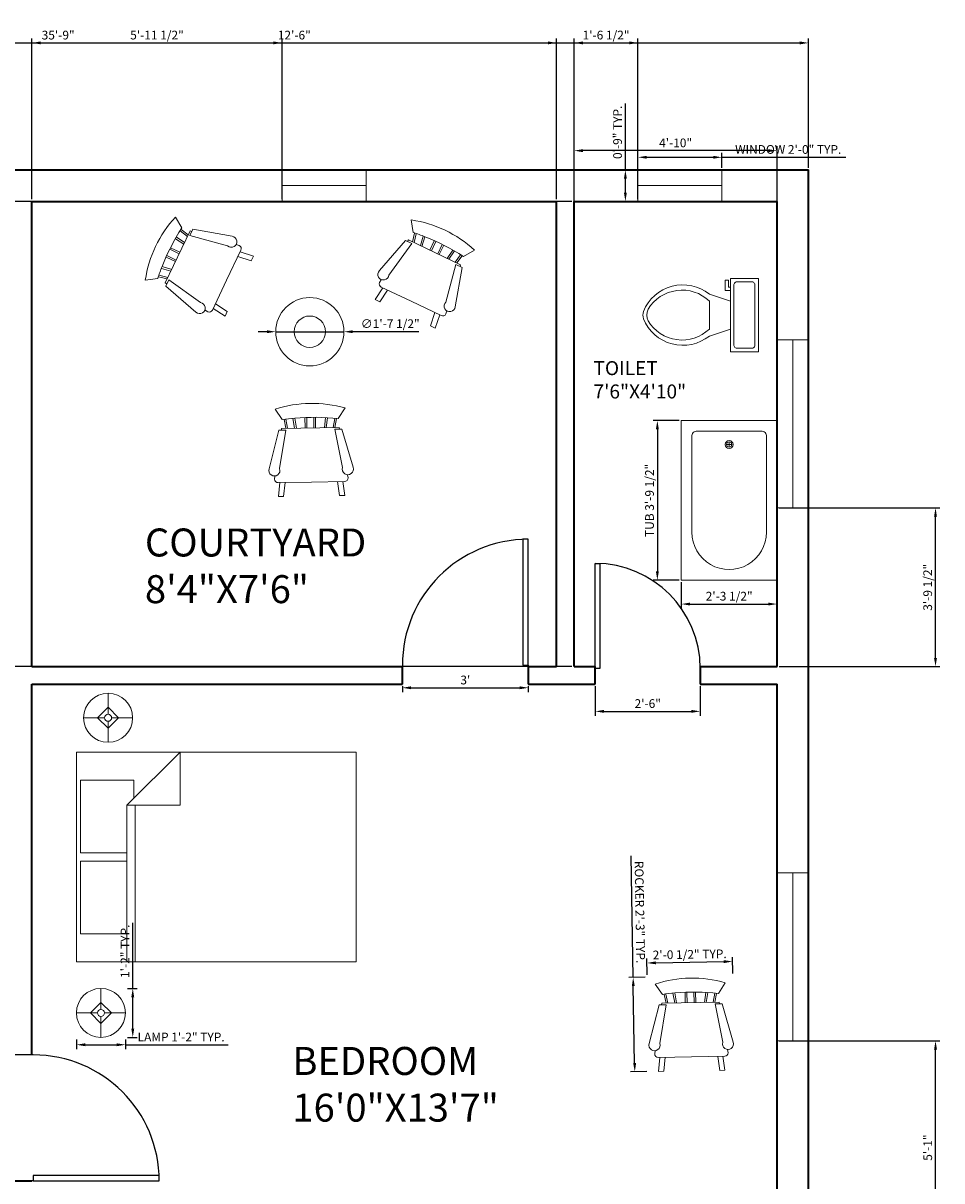
# Model space of a CAD drawing. Units: inches. Extents: x 3715 to 4224, y 2597 to 3354.
# Tile 5 of 5: x 3961 to 4224, y 3023 to 3354. Entities that reach past the tile are written whole.
import ezdxf

# ---------------------------------------------------------------- set-up
doc = ezdxf.new("R2010")
doc.units = ezdxf.units.IN
for name, color, linetype, lineweight in [('A-AREA-IDEN', 4, 'Continuous', 25), ('A-FLOR-FIXT', 9, 'Continuous', 18), ('A-WALL', 7, 'Continuous', 35), ('DIM', 1, 'Continuous', 18), ('DOOR', 3, 'Continuous', 25), ('FURNITURES', 30, 'Continuous', 18), ('WINDOW', 6, 'Continuous', 20)]:
    doc.layers.add(name, color=color, linetype=linetype, lineweight=lineweight)
doc.styles.get("Standard").update_dxf_attribs({"font": 'arial.ttf'})
doc.dimstyles.new('ISO-25', dxfattribs={"dimtxt": 2.5, "dimasz": 2.5, "dimexe": 1.25, "dimexo": 0.625, "dimtad": 1, "dimlunit": 3, "dimtxsty": 'Standard', "dimcen": 2.5, "dimadec": 0, "dimazin": 0, "dimtfac": 1, "dimtmove": 0, "dimatfit": 3, "dimfxl": 1, "dimarcsym": 0})

# ---------------------------------------------------------------- blocks, each defined once
blk = doc.blocks.new('*U4')
for p, q in [((0, 0), (0, -6)), ((-40, 0), (-40, -6))]:
    blk.add_line(p, q)
blk.add_lwpolyline([(0, 0), (0, 40), (-1.75, 40), (-1.75, 0)], close=True)
blk.add_arc((0, 0), 40, 90, 180)
blk = doc.blocks.new('*U2')
for p, q in [((0, 0), (0, -6)), ((40, 0), (40, -6))]:
    blk.add_line(p, q)
blk.add_lwpolyline([(0, 0), (0, 40), (1.75, 40), (1.75, 0)], close=True)
blk.add_arc((0, 0), 40, 0, 90)
blk = doc.blocks.new('Bed - Queen')
for p, q in [((0, -80.00003), (0, 0)), ((0, 0), (59.99999, 0)), ((59.99999, 0), (59.99999, -80.00003)), ((7.99999, -1.2), (28.79998, -1.2)), ((7.99999, -14.4), (7.99999, -1.2)), ((28.79998, -1.2), (28.79998, -14.4)), ((31.19999, -1.2), (51.99999, -1.2)), ((31.19999, -14.4), (31.19999, -1.2)), ((51.99999, -1.2), (51.99999, -16.4)), ((0, -14.4), (44.8, -14.4)), ((59.99999, -29.6), (44.8, -14.4)), ((44.8, -14.4), (44.8, -29.6)), ((51.99999, -16.4), (46.79936, -16.4)), ((44.8, -16.8), (0, -16.8)), ((44.8, -29.6), (59.99999, -29.6)), ((59.99999, -80.00003), (0, -80.00003))]:
    blk.add_line(p, q)
blk = doc.blocks.new('Lamp - Table')
for p, q in [((0, 7), (0, 1)), ((-1, 0), (-7, 0)), ((0, 3), (-3, 0)), ((-3, 0), (0, -3)), ((3, 0), (0, 3)), ((0, -3), (3, 0)), ((1, 0), (7, 0)), ((0, -1), (0, -7))]:
    blk.add_line(p, q)
for radius in [7, 1]:
    blk.add_circle((0, 0), radius)
blk = doc.blocks.new('Toilet - top')
for p, q in [((9.5, -6), (9.5, -2)), ((-10, -8.5), (-8, -8.5)), ((-10, -9.5), (-10, -8.5)), ((-7, -9.5), (-10, -9.5)), ((-8, -8.5), (-8, -8)), ((-7, -8), (-7, -9.5)), ((-4, -8), (-6, -14)), ((4, -8), (6, -14)), ((4, -14), (-4, -14))]:
    blk.add_line(p, q)
blk.add_lwpolyline([(10.5, -8), (10.5, 0), (-10.5, 0), (-10.5, -8)], close=True)
for points in [[(-9.5, -2), (-9.5, -6)], [(8.5, -1), (-8.5, -1)], [(-8.5, -7), (8.5, -7)]]:
    blk.add_lwpolyline(points)
for centre, radius, start, end in [((-8.62, -1.88), 0.884, 81.8699, 188.1301), ((8.62, -1.88), 0.884, 351.8699, 98.1301), ((-8.62, -6.12), 0.884, 171.8699, 278.1301), ((8.62, -6.12), 0.884, 261.8699, 8.1301), ((3.52, -21.58), 12.17, 141.4691, 247.9714), ((4.2, -21.82), 11.33, 136.3677, 238.9468), ((-3.52, -21.58), 12.17, 292.0284, 38.5307), ((-4.2, -21.82), 11.33, 301.053, 43.6321), ((0, -27.88), 4, 245.7318, 294.2682), ((0, -29), 4, 254.8605, 285.1395)]:
    blk.add_arc(centre, radius, start, end)
blk = doc.blocks.new('Bath Tub - 26 x 60 in.')
for p, q in [((9, -17), (9, -19)), ((8, -18), (10, -18))]:
    blk.add_line(p, q)
blk.add_lwpolyline([(0, -36), (0, 0), (60, 0), (60, -36)], close=True)
for points in [[(6, -4), (42, -4)], [(4, -30), (4, -6)], [(42, -32), (6, -32)]]:
    blk.add_lwpolyline(points)
for radius in [1.5, 1]:
    blk.add_circle((9, -18), radius)
for centre, radius, start, end in [((5.75, -5.75), 1.77, 81.8699, 188.1301), ((42, -18), 14, 270, 90), ((5.75, -30.25), 1.77, 171.8699, 278.1301)]:
    blk.add_arc(centre, radius, start, end)
blk = doc.blocks.new('Chair - Rocking')
for p, q in [((-8, -4.5), (-10, -1.5)), ((8, -4.5), (10, -1.5)), ((-7.5, -4.5), (-7, -7)), ((-6.5, -7), (-7.02225, -4.43)), ((-4.5, -7), (-4.96674, -4.19951)), ((-4, -7), (-4.40532, -4.16272)), ((-1.5, -4.05012), (-1.5, -7)), ((-1, -7), (-1, -4.05012)), ((1, -7), (1, -4.04655)), ((1.5, -4.05012), (1.5, -7)), ((4, -7), (4.40187, -4.18694)), ((4.5, -7), (4.96761, -4.19437)), ((6.5, -7), (7, -4.4057)), ((7.5, -4.5), (7, -7)), ((-9, -7.5), (-12, -18.49999)), ((-7, -7.5), (-9, -7.5)), ((-9, -18.49999), (-7, -7.5)), ((-8.23428, -6.99939), (-8.3093, -7.47958)), ((-8.23041, -7), (8.23915, -7)), ((7, -7.5), (9, -7.5)), ((9, -18.49999), (7, -7.5)), ((8.31071, -7.48854), (8.23449, -7.00073)), ((9, -7.5), (12, -18.49999)), ((-10.36644, -20.64523), (-10.5, -21.49999)), ((-9, -22.49999), (-9.5, -26.49999)), ((0, -22.49999), (-9.5, -22.49999)), ((-8, -26.49999), (-7.5, -22.49999)), ((0, -22.49999), (9.5, -22.49999)), ((8, -26.49999), (7.5, -22.49999)), ((9, -22.49999), (9.5, -26.49999)), ((10.5, -21.49999), (10.3575, -20.58798)), ((-9.5, -26.49999), (-8, -26.49999)), ((9.5, -26.49999), (8, -26.49999))]:
    blk.add_line(p, q)
for centre, radius, start, end in [((0, -34.08333), 34.08333, 72.93847, 107.0615), ((0, -68.25004), 64.25, 93.92211, 97.15267), ((0, -68.25004), 64.25, 82.84733, 93.92211), ((-10.5, -18.99999), 1.58114, 161.5651, 18.43495), ((10.5, -18.99999), 1.58114, 161.5651, 18.43495), ((-9.5, -21.49999), 1, 180, 270), ((9.5, -21.49999), 1, 270, 0)]:
    blk.add_arc(centre, radius, start, end)
blk = doc.blocks.new('*D32')
at = {"layer": 'Defpoints', "color": 0, "transparency": 16777216}
for p in [(4069.37, 3164.93), (4105.37, 3164.93), (4105.37, 3163.88)]:
    blk.add_point(p, dxfattribs=at)
at = {"layer": 'DIM', "color": 0, "lineweight": -2, "transparency": 16777216}
for p, q in [((4069.37, 3164.31), (4069.37, 3162.63)), ((4071.87, 3163.88), (4102.87, 3163.88)), ((4105.37, 3164.31), (4105.37, 3162.63))]:
    blk.add_line(p, q, dxfattribs=at)
at = {"layer": 'DIM', "color": 0, "transparency": 16777216}
for points in [[(4071.87, 3164.3), (4071.87, 3163.46), (4069.37, 3163.88)], [(4102.87, 3164.3), (4102.87, 3163.46), (4105.37, 3163.88)]]:
    blk.add_solid(points, dxfattribs=at)
at = {"layer": 'DIM', "color": 0, "transparency": 16777216, "insert": (4087.37, 3165.78), "char_height": 2.5, "attachment_point": 5}
blk.add_mtext("3'", dxfattribs=at)
blk = doc.blocks.new('*D33')
at = {"layer": 'Defpoints', "color": 0, "transparency": 16777216}
for p in [(4124.52, 3164.93), (4154.52, 3164.93), (4154.52, 3157.14)]:
    blk.add_point(p, dxfattribs=at)
at = {"layer": 'DIM', "color": 0, "lineweight": -2, "transparency": 16777216}
for p, q in [((4124.52, 3164.31), (4124.52, 3155.89)), ((4154.52, 3164.31), (4154.52, 3155.89)), ((4127.02, 3157.14), (4152.02, 3157.14))]:
    blk.add_line(p, q, dxfattribs=at)
at = {"layer": 'DIM', "color": 0, "transparency": 16777216}
for points in [[(4127.02, 3157.56), (4127.02, 3156.73), (4124.52, 3157.14)], [(4152.02, 3157.56), (4152.02, 3156.73), (4154.52, 3157.14)]]:
    blk.add_solid(points, dxfattribs=at)
at = {"layer": 'DIM', "color": 0, "transparency": 16777216, "insert": (4139.52, 3159.05), "char_height": 2.5, "attachment_point": 5}
blk.add_mtext('2\'-6"', dxfattribs=at)
blk = doc.blocks.new('*D40')
at = {"layer": 'Defpoints', "color": 0, "transparency": 16777216}
for p in [(4118.48, 3317.43), (4118.48, 3169.93), (4176.48, 3169.93)]:
    blk.add_point(p, dxfattribs=at)
at = {"layer": 'DIM', "color": 0, "lineweight": -2, "transparency": 16777216}
for p, q in [((4118.48, 3170.56), (4118.48, 3318.68)), ((4173.98, 3317.43), (4120.98, 3317.43)), ((4176.48, 3170.56), (4176.48, 3318.68))]:
    blk.add_line(p, q, dxfattribs=at)
at = {"layer": 'DIM', "color": 0, "transparency": 16777216}
for points in [[(4120.98, 3317.85), (4120.98, 3317.01), (4118.48, 3317.43)], [(4173.98, 3317.85), (4173.98, 3317.01), (4176.48, 3317.43)]]:
    blk.add_solid(points, dxfattribs=at)
at = {"layer": 'DIM', "color": 0, "transparency": 16777216, "insert": (4147.48, 3319.33), "char_height": 2.5, "attachment_point": 5}
blk.add_mtext('4\'-10"', dxfattribs=at)
blk = doc.blocks.new('WIN-48IN-9IN-WALL')
blk.add_line((4.5, 48), (4.5, 0))
blk.add_lwpolyline([(0, 48), (9, 48), (9, 0), (0, 0)], close=True)
blk = doc.blocks.new('WIN-24IN-9IN-WALL')
blk.add_line((0, 4.5), (24, 4.5))
blk.add_lwpolyline([(0, 0), (0, 9), (24, 9), (24, 0)], close=True)
blk = doc.blocks.new('*D45')
at = {"layer": 'Defpoints', "color": 0, "transparency": 16777216}
for p in [(4160.73, 3315.53), (4136.73, 3311.93), (4160.73, 3311.93)]:
    blk.add_point(p, dxfattribs=at)
at = {"layer": 'DIM', "color": 0, "lineweight": -2, "transparency": 16777216}
for p, q in [((4136.73, 3312.56), (4136.73, 3316.78)), ((4160.73, 3312.56), (4160.73, 3316.78)), ((4139.23, 3315.53), (4158.23, 3315.53)), ((4160.73, 3315.53), (4196.11, 3315.53))]:
    blk.add_line(p, q, dxfattribs=at)
at = {"layer": 'DIM', "color": 0, "transparency": 16777216}
for points in [[(4139.23, 3315.95), (4139.23, 3315.12), (4136.73, 3315.53)], [(4158.23, 3315.95), (4158.23, 3315.12), (4160.73, 3315.53)]]:
    blk.add_solid(points, dxfattribs=at)
at = {"layer": 'DIM', "color": 0, "transparency": 16777216, "insert": (4179.67, 3317.45), "char_height": 2.5, "attachment_point": 5}
blk.add_mtext('WINDOW 2\'-0" TYP.', dxfattribs=at)
blk = doc.blocks.new('*D46')
at = {"layer": 'Defpoints', "color": 0, "transparency": 16777216}
for p in [(4133.13, 3311.93), (4136.73, 3311.93), (4136.73, 3302.93)]:
    blk.add_point(p, dxfattribs=at)
at = {"layer": 'DIM', "color": 0, "lineweight": -2, "transparency": 16777216}
for p, q in [((4133.13, 3311.93), (4133.13, 3330.92)), ((4136.1, 3311.93), (4131.88, 3311.93)), ((4133.13, 3305.43), (4133.13, 3309.43)), ((4136.1, 3302.93), (4131.88, 3302.93))]:
    blk.add_line(p, q, dxfattribs=at)
at = {"layer": 'DIM', "color": 0, "transparency": 16777216}
for points in [[(4132.71, 3309.43), (4133.54, 3309.43), (4133.13, 3311.93)], [(4132.71, 3305.43), (4133.54, 3305.43), (4133.13, 3302.93)]]:
    blk.add_solid(points, dxfattribs=at)
at = {"layer": 'DIM', "color": 0, "transparency": 16777216, "insert": (4131.22, 3322.68), "char_height": 2.5, "attachment_point": 5, "rotation": 90}
blk.add_mtext('0\'-9" TYP.', dxfattribs=at)
blk = doc.blocks.new('*D47')
at = {"layer": 'Defpoints', "color": 0, "transparency": 16777216}
for p in [(3976.21, 3063.94), (3990.21, 3063.94), (3990.21, 3061.84)]:
    blk.add_point(p, dxfattribs=at)
at = {"layer": 'DIM', "color": 0, "lineweight": -2, "transparency": 16777216}
for p, q in [((3976.21, 3063.31), (3976.21, 3060.59)), ((3978.71, 3061.84), (3987.71, 3061.84)), ((3990.21, 3063.31), (3990.21, 3060.59)), ((3990.21, 3061.84), (4019.56, 3061.84))]:
    blk.add_line(p, q, dxfattribs=at)
at = {"layer": 'DIM', "color": 0, "transparency": 16777216}
for points in [[(3978.71, 3062.25), (3978.71, 3061.42), (3976.21, 3061.84)], [(3987.71, 3062.25), (3987.71, 3061.42), (3990.21, 3061.84)]]:
    blk.add_solid(points, dxfattribs=at)
at = {"layer": 'DIM', "color": 0, "transparency": 16777216, "insert": (4006.13, 3063.72), "char_height": 2.5, "attachment_point": 5}
blk.add_mtext('LAMP 1\'-2" TYP.', dxfattribs=at)
blk = doc.blocks.new('*D48')
at = {"layer": 'Defpoints', "color": 0, "transparency": 16777216}
for p in [(3990.21, 3077.94), (3992.31, 3077.94), (3990.21, 3063.94)]:
    blk.add_point(p, dxfattribs=at)
at = {"layer": 'DIM', "color": 0, "lineweight": -2, "transparency": 16777216}
for p, q in [((3992.31, 3077.94), (3992.31, 3096.69)), ((3990.83, 3077.94), (3993.56, 3077.94)), ((3992.31, 3066.44), (3992.31, 3075.44)), ((3990.83, 3063.94), (3993.56, 3063.94))]:
    blk.add_line(p, q, dxfattribs=at)
at = {"layer": 'DIM', "color": 0, "transparency": 16777216}
for points in [[(3991.89, 3075.44), (3992.72, 3075.44), (3992.31, 3077.94)], [(3991.89, 3066.44), (3992.72, 3066.44), (3992.31, 3063.94)]]:
    blk.add_solid(points, dxfattribs=at)
at = {"layer": 'DIM', "color": 0, "transparency": 16777216, "insert": (3990.42, 3088.56), "char_height": 2.5, "attachment_point": 5, "rotation": 90}
blk.add_mtext('1\'-2" TYP.', dxfattribs=at)
blk = doc.blocks.new('*D49')
at = {"layer": 'Defpoints', "color": 0, "transparency": 16777216}
for p in [(4139.39, 3081.17), (4135.35, 3081.09), (4139.87, 3054.17)]:
    blk.add_point(p, dxfattribs=at)
at = {"layer": 'DIM', "color": 0, "lineweight": -2, "transparency": 16777216}
for p, q in [((4135.35, 3081.09), (4134.74, 3115.86)), ((4138.77, 3081.15), (4134.1, 3081.07)), ((4135.77, 3056.6), (4135.39, 3078.59)), ((4139.24, 3054.16), (4134.57, 3054.08))]:
    blk.add_line(p, q, dxfattribs=at)
at = {"layer": 'DIM', "color": 0, "transparency": 16777216}
for points in [[(4135.81, 3078.6), (4134.97, 3078.59), (4135.35, 3081.09)], [(4136.19, 3056.61), (4135.36, 3056.59), (4135.82, 3054.1)]]:
    blk.add_solid(points, dxfattribs=at)
at = {"layer": 'DIM', "color": 0, "transparency": 16777216, "insert": (4136.94, 3099.76), "char_height": 2.5, "attachment_point": 5, "rotation": 271.0049}
blk.add_mtext('ROCKER 2\'-3" TYP.', dxfattribs=at)
blk = doc.blocks.new('*D50')
at = {"layer": 'Defpoints', "color": 0, "transparency": 16777216}
for p in [(4163.75, 3085.64), (4139.39, 3081.17), (4163.83, 3081.59)]:
    blk.add_point(p, dxfattribs=at)
at = {"layer": 'DIM', "color": 0, "lineweight": -2, "transparency": 16777216}
for p, q in [((4139.38, 3081.79), (4139.3, 3086.46)), ((4141.82, 3085.26), (4161.26, 3085.6)), ((4163.81, 3082.22), (4163.73, 3086.89))]:
    blk.add_line(p, q, dxfattribs=at)
at = {"layer": 'DIM', "color": 0, "transparency": 16777216}
for points in [[(4141.82, 3085.68), (4141.83, 3084.84), (4139.32, 3085.21)], [(4161.25, 3086.02), (4161.26, 3085.18), (4163.75, 3085.64)]]:
    blk.add_solid(points, dxfattribs=at)
at = {"layer": 'DIM', "color": 0, "transparency": 16777216, "insert": (4151.51, 3087.35), "char_height": 2.5, "attachment_point": 5, "rotation": 1.0049}
blk.add_mtext('2\'-0 1/2" TYP.', dxfattribs=at)
blk = doc.blocks.new('*D71')
at = {"layer": 'Defpoints', "color": 0, "transparency": 16777216}
for p in [(4149.11, 3240.27), (4142.27, 3194.66), (4149.11, 3194.66)]:
    blk.add_point(p, dxfattribs=at)
at = {"layer": 'DIM', "color": 0, "lineweight": -2, "transparency": 16777216}
for p, q in [((4148.49, 3240.27), (4141.02, 3240.27)), ((4142.27, 3237.77), (4142.27, 3197.16)), ((4148.49, 3194.66), (4141.02, 3194.66))]:
    blk.add_line(p, q, dxfattribs=at)
at = {"layer": 'DIM', "color": 0, "transparency": 16777216}
for points in [[(4141.85, 3237.77), (4142.69, 3237.77), (4142.27, 3240.27)], [(4141.85, 3197.16), (4142.69, 3197.16), (4142.27, 3194.66)]]:
    blk.add_solid(points, dxfattribs=at)
at = {"layer": 'DIM', "color": 0, "transparency": 16777216, "insert": (4140.35, 3217.46), "char_height": 2.5, "attachment_point": 5, "rotation": 90}
blk.add_mtext('TUB 3\'-9 1/2"', dxfattribs=at)
blk = doc.blocks.new('*D72')
at = {"layer": 'Defpoints', "color": 0, "transparency": 16777216}
for p in [(4149.11, 3194.66), (4176.48, 3194.66), (4176.48, 3187.82)]:
    blk.add_point(p, dxfattribs=at)
at = {"layer": 'DIM', "color": 0, "lineweight": -2, "transparency": 16777216}
for p, q in [((4149.11, 3194.03), (4149.11, 3186.57)), ((4176.48, 3194.03), (4176.48, 3186.57)), ((4151.61, 3187.82), (4173.98, 3187.82))]:
    blk.add_line(p, q, dxfattribs=at)
at = {"layer": 'DIM', "color": 0, "transparency": 16777216}
for points in [[(4151.61, 3188.24), (4151.61, 3187.4), (4149.11, 3187.82)], [(4173.98, 3188.24), (4173.98, 3187.4), (4176.48, 3187.82)]]:
    blk.add_solid(points, dxfattribs=at)
at = {"layer": 'DIM', "color": 0, "transparency": 16777216, "insert": (4162.79, 3189.74), "char_height": 2.5, "attachment_point": 5}
blk.add_mtext('2\'-3 1/2"', dxfattribs=at)
blk = doc.blocks.new('*D75')
at = {"layer": 'Defpoints', "color": 0, "transparency": 16777216}
for p in [(4185.48, 3348.23), (3756.48, 3311.93), (4185.48, 3311.93)]:
    blk.add_point(p, dxfattribs=at)
at = {"layer": 'DIM', "color": 0, "lineweight": -2, "transparency": 16777216}
for p, q in [((3756.48, 3312.56), (3756.48, 3349.48)), ((4185.48, 3312.56), (4185.48, 3349.48)), ((3758.98, 3348.23), (4182.98, 3348.23))]:
    blk.add_line(p, q, dxfattribs=at)
at = {"layer": 'DIM', "color": 0, "transparency": 16777216}
for points in [[(3758.98, 3348.65), (3758.98, 3347.82), (3756.48, 3348.23)], [(4182.98, 3348.65), (4182.98, 3347.82), (4185.48, 3348.23)]]:
    blk.add_solid(points, dxfattribs=at)
at = {"layer": 'DIM', "color": 0, "transparency": 16777216, "insert": (3970.98, 3350.14), "char_height": 2.5, "attachment_point": 5}
blk.add_mtext('35\'-9"', dxfattribs=at)
blk = doc.blocks.new('*D77')
at = {"layer": 'Defpoints', "color": 0, "transparency": 16777216}
for p in [(3720.18, 3302.93), (4118.48, 3302.93), (4118.48, 3169.93)]:
    blk.add_point(p, dxfattribs=at)
at = {"layer": 'DIM', "color": 0, "lineweight": -2, "transparency": 16777216}
for p, q in [((4117.85, 3302.93), (3718.93, 3302.93)), ((3720.18, 3172.43), (3720.18, 3300.43)), ((4117.85, 3169.93), (3718.93, 3169.93))]:
    blk.add_line(p, q, dxfattribs=at)
at = {"layer": 'DIM', "color": 0, "transparency": 16777216}
for points in [[(3719.76, 3300.43), (3720.59, 3300.43), (3720.18, 3302.93)], [(3719.76, 3172.43), (3720.59, 3172.43), (3720.18, 3169.93)]]:
    blk.add_solid(points, dxfattribs=at)
at = {"layer": 'DIM', "color": 0, "transparency": 16777216, "insert": (3718.3, 3236.43), "char_height": 2.5, "attachment_point": 5, "rotation": 90}
blk.add_mtext('11\'-1"', dxfattribs=at)
blk = doc.blocks.new('*D78')
at = {"layer": 'Defpoints', "color": 0, "transparency": 16777216}
for p in [(4113.48, 3348.23), (3963.48, 3302.93), (4113.48, 3302.93)]:
    blk.add_point(p, dxfattribs=at)
at = {"layer": 'DIM', "color": 0, "lineweight": -2, "transparency": 16777216}
for p, q in [((3963.48, 3303.56), (3963.48, 3349.48)), ((4113.48, 3303.56), (4113.48, 3349.48)), ((3965.98, 3348.23), (4110.98, 3348.23))]:
    blk.add_line(p, q, dxfattribs=at)
at = {"layer": 'DIM', "color": 0, "transparency": 16777216}
for points in [[(3965.98, 3348.65), (3965.98, 3347.82), (3963.48, 3348.23)], [(4110.98, 3348.65), (4110.98, 3347.82), (4113.48, 3348.23)]]:
    blk.add_solid(points, dxfattribs=at)
at = {"layer": 'DIM', "color": 0, "transparency": 16777216, "insert": (4038.48, 3350.14), "char_height": 2.5, "attachment_point": 5}
blk.add_mtext('12\'-6"', dxfattribs=at)
blk = doc.blocks.new('*D87')
at = {"layer": 'Defpoints', "color": 0, "transparency": 16777216}
for p in [(4176.48, 3062.95), (4221.78, 3062.95), (4185.48, 3001.93)]:
    blk.add_point(p, dxfattribs=at)
at = {"layer": 'DIM', "color": 0, "lineweight": -2, "transparency": 16777216}
for p, q in [((4177.1, 3062.95), (4223.03, 3062.95)), ((4221.78, 3004.43), (4221.78, 3060.45)), ((4186.1, 3001.93), (4223.03, 3001.93))]:
    blk.add_line(p, q, dxfattribs=at)
at = {"layer": 'DIM', "color": 0, "transparency": 16777216}
for points in [[(4221.36, 3060.45), (4222.19, 3060.45), (4221.78, 3062.95)], [(4221.36, 3004.43), (4222.19, 3004.43), (4221.78, 3001.93)]]:
    blk.add_solid(points, dxfattribs=at)
at = {"layer": 'DIM', "color": 0, "transparency": 16777216, "insert": (4219.87, 3032.44), "char_height": 2.5, "attachment_point": 5, "rotation": 90}
blk.add_mtext('5\'-1"', dxfattribs=at)
blk = doc.blocks.new('*D88')
at = {"layer": 'Defpoints', "color": 0, "transparency": 16777216}
for p in [(4176.48, 3215.3), (4221.78, 3215.3), (4176.48, 3169.93)]:
    blk.add_point(p, dxfattribs=at)
at = {"layer": 'DIM', "color": 0, "lineweight": -2, "transparency": 16777216}
for p, q in [((4177.1, 3215.3), (4223.03, 3215.3)), ((4221.78, 3172.43), (4221.78, 3212.8)), ((4177.1, 3169.93), (4223.03, 3169.93))]:
    blk.add_line(p, q, dxfattribs=at)
at = {"layer": 'DIM', "color": 0, "transparency": 16777216}
for points in [[(4221.36, 3212.8), (4222.19, 3212.8), (4221.78, 3215.3)], [(4221.36, 3172.43), (4222.19, 3172.43), (4221.78, 3169.93)]]:
    blk.add_solid(points, dxfattribs=at)
at = {"layer": 'DIM', "color": 0, "transparency": 16777216, "insert": (4219.86, 3192.62), "char_height": 2.5, "attachment_point": 5, "rotation": 90}
blk.add_mtext('3\'-9 1/2"', dxfattribs=at)
blk = doc.blocks.new('*D90')
at = {"layer": 'Defpoints', "color": 0, "transparency": 16777216}
for p in [(3720.18, 3022.93), (3963.48, 3022.93), (3963.48, 3001.93)]:
    blk.add_point(p, dxfattribs=at)
at = {"layer": 'DIM', "color": 0, "lineweight": -2, "transparency": 16777216}
for p, q in [((3962.85, 3022.93), (3718.93, 3022.93)), ((3720.18, 3004.43), (3720.18, 3020.43)), ((3962.85, 3001.93), (3718.93, 3001.93))]:
    blk.add_line(p, q, dxfattribs=at)
at = {"layer": 'DIM', "color": 0, "transparency": 16777216}
for points in [[(3719.76, 3020.43), (3720.59, 3020.43), (3720.18, 3022.93)], [(3719.76, 3004.43), (3720.59, 3004.43), (3720.18, 3001.93)]]:
    blk.add_solid(points, dxfattribs=at)
at = {"layer": 'DIM', "color": 0, "transparency": 16777216, "insert": (3718.27, 3012.43), "char_height": 2.5, "attachment_point": 5, "rotation": 90}
blk.add_mtext('1\'-9"', dxfattribs=at)
blk = doc.blocks.new('*D95')
at = {"layer": 'Defpoints', "color": 0, "transparency": 16777216}
for p in [(4034.98, 3348.23), (3963.48, 3302.93), (4034.98, 3302.93)]:
    blk.add_point(p, dxfattribs=at)
at = {"layer": 'DIM', "color": 0, "lineweight": -2, "transparency": 16777216}
for p, q in [((3963.48, 3303.56), (3963.48, 3349.48)), ((4034.98, 3303.56), (4034.98, 3349.48)), ((3965.98, 3348.23), (4032.48, 3348.23))]:
    blk.add_line(p, q, dxfattribs=at)
at = {"layer": 'DIM', "color": 0, "transparency": 16777216}
for points in [[(3965.98, 3348.65), (3965.98, 3347.82), (3963.48, 3348.23)], [(4032.48, 3348.65), (4032.48, 3347.82), (4034.98, 3348.23)]]:
    blk.add_solid(points, dxfattribs=at)
at = {"layer": 'DIM', "color": 0, "transparency": 16777216, "insert": (3999.23, 3350.15), "char_height": 2.5, "attachment_point": 5}
blk.add_mtext('5\'-11 1/2"', dxfattribs=at)
blk = doc.blocks.new('*D96')
at = {"layer": 'Defpoints', "color": 0, "transparency": 16777216}
for p in [(4136.73, 3348.23), (4118.48, 3302.93), (4136.73, 3302.93)]:
    blk.add_point(p, dxfattribs=at)
at = {"layer": 'DIM', "color": 0, "lineweight": -2, "transparency": 16777216}
for p, q in [((4118.48, 3303.56), (4118.48, 3349.48)), ((4136.73, 3303.56), (4136.73, 3349.48)), ((4120.98, 3348.23), (4134.23, 3348.23))]:
    blk.add_line(p, q, dxfattribs=at)
at = {"layer": 'DIM', "color": 0, "transparency": 16777216}
for points in [[(4120.98, 3348.65), (4120.98, 3347.82), (4118.48, 3348.23)], [(4134.23, 3348.65), (4134.23, 3347.82), (4136.73, 3348.23)]]:
    blk.add_solid(points, dxfattribs=at)
at = {"layer": 'DIM', "color": 0, "transparency": 16777216, "insert": (4127.6, 3350.15), "char_height": 2.5, "attachment_point": 5}
blk.add_mtext('1\'-6 1/2"', dxfattribs=at)
blk = doc.blocks.new('*D102')
at = {"layer": 'Defpoints', "color": 0, "transparency": 16777216}
for p in [(4033.16, 3265.67), (4052.68, 3265.67)]:
    blk.add_point(p, dxfattribs=at)
at = {"layer": 'DIM', "color": 0, "lineweight": -2, "transparency": 16777216}
for p, q in [((4030.66, 3265.67), (4028.16, 3265.67)), ((4033.16, 3265.67), (4052.68, 3265.67)), ((4074.12, 3265.67), (4055.18, 3265.67))]:
    blk.add_line(p, q, dxfattribs=at)
at = {"layer": 'DIM', "color": 0, "transparency": 16777216}
for points in [[(4030.66, 3266.08), (4030.66, 3265.25), (4033.16, 3265.67)], [(4055.18, 3266.08), (4055.18, 3265.25), (4052.68, 3265.67)]]:
    blk.add_solid(points, dxfattribs=at)
at = {"layer": 'DIM', "color": 0, "transparency": 16777216, "insert": (4065.9, 3267.64), "char_height": 2.5, "attachment_point": 5, "rotation": 0.0022}
blk.add_mtext('∅1\'-7 1/2"', dxfattribs=at)

msp = doc.modelspace()

# ---------------------------------------------------------------- linework, layer by layer
at = {"layer": 'A-WALL'}
for p, q in [((3756.476, 3311.934), (4185.476, 3311.934)), ((4185.476, 2634.934), (4185.476, 3311.934)), ((3963.476, 3302.934), (4113.476, 3302.934)), ((3963.476, 3169.934), (3963.476, 3302.934)), ((4113.476, 3169.934), (4113.476, 3302.934)), ((4118.476, 3169.934), (4118.476, 3302.934)), ((4118.476, 3302.934), (4176.476, 3302.934)), ((4176.476, 3169.934), (4176.476, 3302.934)), ((3963.476, 3169.934), (4069.374, 3169.934)), ((4105.374, 3169.934), (4113.476, 3169.934)), ((4118.476, 3169.934), (4124.523, 3169.934)), ((4154.523, 3169.934), (4176.476, 3169.934)), ((3963.476, 3164.934), (4069.374, 3164.934)), ((3963.476, 3058.934), (3963.476, 3164.934)), ((4105.374, 3164.934), (4124.523, 3164.934)), ((4154.523, 3164.934), (4176.476, 3164.934)), ((4176.476, 2833.934), (4176.476, 3164.934)), ((3958.476, 3022.934), (3963.476, 3022.934))]:
    msp.add_line(p, q, dxfattribs=at)
for points in [[(4069.374, 3164.934), (4069.374, 3169.934)], [(4105.374, 3169.934), (4105.374, 3164.934)], [(4124.523, 3164.934), (4124.523, 3169.934)], [(4154.523, 3169.934), (4154.523, 3164.934)]]:
    msp.add_lwpolyline(points, dxfattribs=at)
at = {"layer": 'FURNITURES'}
for radius in [9.763, 4.493]:
    msp.add_circle((4042.92, 3265.668), radius, dxfattribs=at)

# ---------------------------------------------------------------- block references
at = {"layer": 'A-FLOR-FIXT', "rotation": 270}
msp.add_blockref('Toilet - top', (4171.144, 3270.428), dxfattribs=at)
at = {"layer": 'A-FLOR-FIXT', "xscale": 0.760116950066092, "yscale": 0.760116950066092, "zscale": 0.760116950066092, "rotation": 270}
msp.add_blockref('Bath Tub - 26 x 60 in.', (4176.476, 3240.267), dxfattribs=at)
at = {"layer": 'DOOR'}
for name, p, xscale, yscale, zscale in [('*U4', (4105.374, 3170.334), 0.9, 0.9, 0.9), ('*U2', (4124.523, 3169.434), 0.75, 0.75, 0.75)]:
    msp.add_blockref(name, p, dxfattribs=dict(at, xscale=xscale, yscale=yscale, zscale=zscale))
at = {"layer": 'DOOR', "xscale": 0.9, "yscale": 0.9, "zscale": 0.9, "rotation": 270}
msp.add_blockref('*U4', (3963.876, 3022.934), dxfattribs=at)
at = {"layer": 'FURNITURES'}
for name, p, rotation in [('Chair - Rocking', (3998.833, 3290.077), 64.53664434740696), ('Chair - Rocking', (4081.591, 3294.679), 334.536644347407), ('Chair - Rocking', (4042.96, 3245.19), 1.004886468457085), ('Bed - Queen', (3976.215, 3085.515), 90), ('Chair - Rocking', (4151.619, 3080.88), 1.004886468457085)]:
    msp.add_blockref(name, p, dxfattribs=dict(at, rotation=rotation))
for p in [(3985.265, 3155.3), (3983.205, 3070.937)]:
    msp.add_blockref('Lamp - Table', p, dxfattribs=at)
at = {"layer": 'WINDOW'}
for name, p in [('WIN-24IN-9IN-WALL', (4034.98, 3302.934)), ('WIN-24IN-9IN-WALL', (4136.726, 3302.934)), ('WIN-48IN-9IN-WALL', (4176.476, 3215.305)), ('WIN-48IN-9IN-WALL', (4176.476, 3062.946))]:
    msp.add_blockref(name, p, dxfattribs=at)

# ---------------------------------------------------------------- texts
at = {"layer": 'A-AREA-IDEN', "attachment_point": 1}
for s, insert, char_height in [('TOILET\\P7\'6"X4\'10"', (4124.015, 3257.254), 4), ('COURTYARD\\P8\'4"X7\'6"', (3995.778, 3209.416), 8), ('BEDROOM\\P16\'0"X13\'7"', (4037.94, 3061.203), 8)]:
    msp.add_mtext_dynamic_manual_height_columns(s, width=94.29963, gutter_width=12.5, heights=[0], dxfattribs=dict(at, insert=insert, char_height=char_height))

# ---------------------------------------------------------------- dimensions: what is measured, and where the dimension line sits
at = {"layer": 'DIM'}
for base, p1, p2, override, picture, middle in [((4034.979, 3348.234), (3963.476, 3302.934), (4034.979, 3302.934), {"dimdec": 1, "dimlfac": 1, "dimrnd": 0, "dimzin": 1, "dimdsep": 46, "dimlunit": 4, "dimfrac": 2}, '*D95', (3999.227, 3350.151)), ((4136.7256, 3348.2337), (4118.4755, 3302.9337), (4136.7256, 3302.9337), {"dimdec": 1, "dimlfac": 1, "dimrnd": 0, "dimzin": 1, "dimdsep": 46, "dimlunit": 4, "dimfrac": 2}, '*D96', (4127.6006, 3350.1513)), ((4185.476, 3348.234), (3756.476, 3311.934), (4185.476, 3311.934), {"dimdec": 1, "dimlfac": 1, "dimrnd": 0, "dimzin": 1, "dimdsep": 46, "dimlunit": 4, "dimfrac": 2}, '*D75', (3970.976, 3350.136)), ((4113.476, 3348.234), (3963.476, 3302.934), (4113.476, 3302.934), {"dimdec": 1, "dimlfac": 1, "dimrnd": 0, "dimzin": 1, "dimdsep": 46, "dimlunit": 4, "dimfrac": 2}, '*D78', (4038.476, 3350.135)), ((4118.476, 3317.43), (4176.476, 3169.934), (4118.476, 3169.934), {"dimclrd": 0, "dimclre": 0, "dimclrt": 0}, '*D40', (4147.476, 3319.332)), ((4176.476, 3187.819), (4149.111, 3194.66), (4176.476, 3194.66), {"dimdec": 1, "dimlfac": 1, "dimrnd": 0, "dimzin": 1, "dimdsep": 46, "dimlunit": 4, "dimfrac": 2}, '*D72', (4162.793, 3189.737)), ((4105.374, 3163.88), (4069.374, 3164.934), (4105.374, 3164.934), {"dimclrd": 0, "dimclre": 0, "dimclrt": 0}, '*D32', (4087.374, 3165.783)), ((4154.523, 3157.144), (4124.523, 3164.934), (4154.523, 3164.934), {"dimclrd": 0, "dimclre": 0, "dimclrt": 0}, '*D33', (4139.523, 3159.045))]:
    dim = msp.add_linear_dim(base=base, p1=p1, p2=p2, dimstyle='ISO-25', override=override, dxfattribs=at)
    dim.commit()
    dim.dimension.update_dxf_attribs({"geometry": picture, "text_midpoint": middle})
for base, p1, p2, angle, text, picture, middle in [((4133.126, 3311.934), (4136.726, 3302.934), (4136.726, 3311.934), 90, '<> TYP.', '*D46', (4131.224, 3322.678)), ((4142.27, 3194.66), (4149.111, 3240.267), (4149.111, 3194.66), 270, 'TUB <>', '*D71', (4140.352, 3217.463)), ((4135.345, 3081.094), (4139.868, 3054.17), (4139.395, 3081.165), 91.00489, 'ROCKER <> TYP.', '*D49', (4136.937, 3099.761)), ((3992.305, 3077.937), (3990.205, 3063.937), (3990.205, 3077.937), 90, '<> TYP.', '*D48', (3990.424, 3088.564)), ((4163.755, 3085.643), (4139.395, 3081.165), (4163.826, 3081.594), 1.00489, '<> TYP.', '*D50', (4151.506, 3087.346))]:
    dim = msp.add_linear_dim(base=base, p1=p1, p2=p2, angle=angle, text=text, dimstyle='ISO-25', override={"dimdec": 1, "dimlfac": 1, "dimrnd": 0, "dimzin": 1, "dimdsep": 46, "dimlunit": 4, "dimfrac": 2}, dxfattribs=at)
    dim.commit()
    dim.dimension.update_dxf_attribs({"geometry": picture, "text_midpoint": middle})
for base, p1, p2, text, picture, middle in [((4160.726, 3315.534), (4136.726, 3311.934), (4160.726, 3311.934), 'WINDOW <> TYP.', '*D45', (4179.668, 3317.452)), ((3990.205, 3061.837), (3976.205, 3063.937), (3990.205, 3063.937), 'LAMP <> TYP.', '*D47', (4006.135, 3063.718))]:
    dim = msp.add_linear_dim(base=base, p1=p1, p2=p2, text=text, dimstyle='ISO-25', override={"dimdec": 1, "dimlfac": 1, "dimrnd": 0, "dimzin": 1, "dimdsep": 46, "dimlunit": 4, "dimfrac": 2}, dxfattribs=at)
    dim.commit()
    dim.dimension.update_dxf_attribs({"geometry": picture, "text_midpoint": middle})
for base, p1, p2, picture, middle in [((3720.176, 3302.934), (4118.476, 3169.934), (4118.476, 3302.934), '*D77', (3718.295, 3236.434)), ((4221.776, 3215.305), (4176.476, 3169.934), (4176.476, 3215.305), '*D88', (4219.857, 3192.619)), ((4221.776, 3062.946), (4185.476, 3001.934), (4176.476, 3062.946), '*D87', (4219.874, 3032.44)), ((3720.176, 3022.934), (3963.476, 3001.934), (3963.476, 3022.934), '*D90', (3718.274, 3012.434))]:
    dim = msp.add_linear_dim(base=base, p1=p1, p2=p2, angle=90, dimstyle='ISO-25', override={"dimdec": 1, "dimlfac": 1, "dimrnd": 0, "dimzin": 1, "dimdsep": 46, "dimlunit": 4, "dimfrac": 2}, dxfattribs=at)
    dim.commit()
    dim.dimension.update_dxf_attribs({"geometry": picture, "text_midpoint": middle})
dim = msp.add_diameter_dim_2p(p1=(4033.157, 3265.667), p2=(4052.683, 3265.668), dimstyle='ISO-25', override={"dimdec": 1, "dimlfac": 1, "dimrnd": 0, "dimzin": 1, "dimdsep": 46, "dimlunit": 4, "dimfrac": 2}, dxfattribs=at)
dim.commit()
dim.dimension.update_dxf_attribs({"geometry": '*D102', "text_midpoint": (4065.903, 3265.668), "dimtype": 163})

doc.saveas('drawing.dxf')
